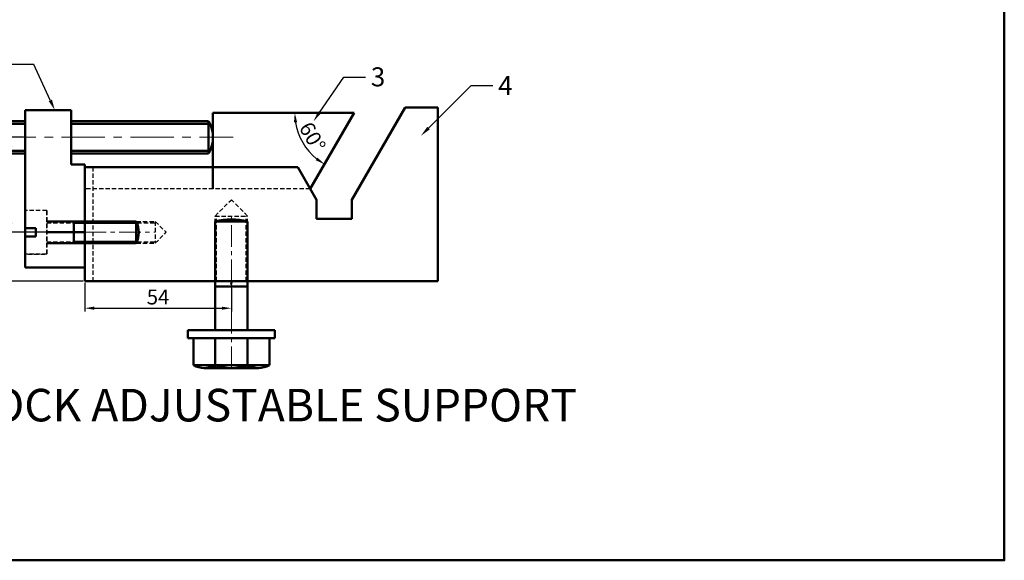
# Model space of a CAD drawing. Units: millimetres. Extents: x 10 to 613, y -226 to 271.
# Tile 2 of 4: x 251 to 613, y -226 to -26. Entities that reach past the tile are written whole.
import ezdxf
from ezdxf import colors
from ezdxf.entities.mleader import LeaderData, LeaderLine
from ezdxf.math import Vec2, Vec3

# ---------------------------------------------------------------- set-up
doc = ezdxf.new("R2010")
doc.units = ezdxf.units.MM
doc.header["$LTSCALE"] = 0.5
doc.linetypes.add('CENTER', pattern=[50.8, 31.75, -6.35, 6.35, -6.35])
doc.linetypes.add('HIDDEN', pattern=[9.525, 6.35, -3.175])
for name, color, linetype, lineweight in [('M-CNTR', 1, 'CENTER', 18), ('M-DIMS', 2, 'Continuous', 25), ('M-HIDN', 6, 'HIDDEN', 25), ('M-OUTL', 7, 'Continuous', 50), ('M-TEXT', 3, 'Continuous', 25), ('M-TTLB', 7, 'Continuous', 50)]:
    doc.layers.add(name, color=color, linetype=linetype, lineweight=lineweight)
doc.styles.get("Standard").update_dxf_attribs({"font": 'arial.ttf'})
doc.dimstyles.new('ISO-25', dxfattribs={"dimtxt": 5.5, "dimasz": 3.5, "dimexe": 1.25, "dimexo": 0.625, "dimtad": 1, "dimtoh": 1, "dimtxsty": 'Standard', "dimcen": 2.5, "dimadec": 0, "dimazin": 0, "dimtfac": 1, "dimtmove": 0, "dimatfit": 3, "dimfxl": 1, "dimarcsym": 0})

# ---------------------------------------------------------------- blocks, each defined once
blk = doc.blocks.new('*D52')
at = {"layer": 'Defpoints', "color": 0, "ltscale": 0.5, "transparency": 16777216}
for p in [(274.69, -104.71), (238.97, -122.71), (274.69, -122.71)]:
    blk.add_point(p, dxfattribs=at)
at = {"layer": 'M-DIMS', "color": 0, "lineweight": -2, "ltscale": 0.5, "transparency": 16777216}
for p, q in [((274.07, -104.71), (237.72, -104.71)), ((238.97, -108.21), (238.97, -119.21)), ((274.07, -122.71), (237.72, -122.71))]:
    blk.add_line(p, q, dxfattribs=at)
at = {"layer": 'M-DIMS', "color": 0, "ltscale": 0.5, "transparency": 16777216}
for points in [[(238.39, -108.21), (239.56, -108.21), (238.97, -104.71)], [(238.39, -119.21), (239.56, -119.21), (238.97, -122.71)]]:
    blk.add_solid(points, dxfattribs=at)
at = {"layer": 'M-DIMS', "color": 0, "ltscale": 0.5, "transparency": 16777216, "insert": (235.54, -113.71), "char_height": 5.5, "attachment_point": 5, "rotation": 90}
blk.add_mtext('18', dxfattribs=at)
blk = doc.blocks.new('*D53')
at = {"layer": 'Defpoints', "color": 0, "ltscale": 0.5, "transparency": 16777216}
for p in [(252.69, -69.71), (247.41, -104.71), (252.69, -104.71)]:
    blk.add_point(p, dxfattribs=at)
at = {"layer": 'M-DIMS', "color": 0, "lineweight": -2, "ltscale": 0.5, "transparency": 16777216}
for p, q in [((252.07, -69.71), (246.16, -69.71)), ((247.41, -73.21), (247.41, -101.21)), ((252.07, -104.71), (246.16, -104.71))]:
    blk.add_line(p, q, dxfattribs=at)
at = {"layer": 'M-DIMS', "color": 0, "ltscale": 0.5, "transparency": 16777216}
for points in [[(246.83, -73.21), (247.99, -73.21), (247.41, -69.71)], [(246.83, -101.21), (247.99, -101.21), (247.41, -104.71)]]:
    blk.add_solid(points, dxfattribs=at)
at = {"layer": 'M-DIMS', "color": 0, "ltscale": 0.5, "transparency": 16777216, "insert": (243.98, -87.21), "char_height": 5.5, "attachment_point": 5, "rotation": 90}
blk.add_mtext('35', dxfattribs=at)
blk = doc.blocks.new('*D54')
at = {"layer": 'Defpoints', "color": 0, "ltscale": 0.5, "transparency": 16777216}
for p in [(274.69, -122.71), (328.69, -124.69), (328.69, -132.66)]:
    blk.add_point(p, dxfattribs=at)
at = {"layer": 'M-DIMS', "color": 0, "lineweight": -2, "ltscale": 0.5, "transparency": 16777216}
for p, q in [((274.69, -123.33), (274.69, -133.91)), ((328.69, -125.31), (328.69, -133.91)), ((278.19, -132.66), (325.19, -132.66))]:
    blk.add_line(p, q, dxfattribs=at)
at = {"layer": 'M-DIMS', "color": 0, "ltscale": 0.5, "transparency": 16777216}
for points in [[(278.19, -132.08), (278.19, -133.24), (274.69, -132.66)], [(325.19, -132.08), (325.19, -133.24), (328.69, -132.66)]]:
    blk.add_solid(points, dxfattribs=at)
at = {"layer": 'M-DIMS', "color": 0, "ltscale": 0.5, "transparency": 16777216, "insert": (301.69, -129.24), "char_height": 5.5, "attachment_point": 5}
blk.add_mtext('54', dxfattribs=at)
blk = doc.blocks.new('*D55')
at = {"layer": 'Defpoints', "color": 0, "ltscale": 0.5, "transparency": 16777216}
for p in [(321.92, -60.71), (373.92, -60.71), (373.92, -60.71), (353.37, -68.19), (357.75, -88.71)]:
    blk.add_point(p, dxfattribs=at)
at = {"layer": 'M-DIMS', "color": 0, "lineweight": -2, "ltscale": 0.5, "transparency": 16777216}
blk.add_arc((373.92, -60.71), 21.87, 189.1792, 230.8208, dxfattribs=at)
at = {"layer": 'M-DIMS', "color": 0, "ltscale": 0.5, "transparency": 16777216}
for points in [[(351.75, -64.24), (352.91, -64.15), (352.05, -60.71)], [(360.43, -77.18), (359.77, -78.14), (362.98, -79.65)]]:
    blk.add_solid(points, dxfattribs=at)
at = {"layer": 'M-DIMS', "color": 0, "ltscale": 0.5, "transparency": 16777216, "insert": (357.95, -69.93), "char_height": 5.5, "attachment_point": 5, "rotation": 300}
blk.add_mtext('60°', dxfattribs=at)

msp = doc.modelspace()

# ---------------------------------------------------------------- linework, layer by layer
at = {"layer": 'M-CNTR'}
msp.add_line((215.384, -69.708), (329.34, -69.708), dxfattribs=at)
at = {"layer": 'M-CNTR', "ltscale": 0.5}
for p, q in [((328.691, -122.708), (328.691, -98.708)), ((274.691, -104.708), (300.691, -104.708)), ((328.691, -154.69), (328.691, -122.977))]:
    msp.add_line(p, q, dxfattribs=at)
at = {"layer": 'M-HIDN', "ltscale": 0.5}
for p, q in [((277.691, -80.708), (277.691, -122.708)), ((357.752, -88.708), (274.691, -88.708)), ((322.691, -98.708), (328.691, -92.708)), ((334.691, -98.708), (328.691, -92.708)), ((260.691, -96.708), (252.691, -96.708)), ((260.691, -96.708), (253.691, -96.708)), ((260.691, -96.708), (260.691, -112.708)), ((260.691, -112.708), (260.691, -96.708)), ((274.691, -100.708), (260.691, -100.708)), ((260.691, -101.208), (300.691, -101.208)), ((274.691, -100.708), (300.691, -100.708)), ((300.691, -100.708), (300.691, -108.708)), ((300.691, -100.708), (304.691, -104.708)), ((322.691, -122.708), (322.691, -98.708)), ((322.691, -98.708), (334.691, -98.708)), ((323.191, -122.708), (323.191, -98.708)), ((334.191, -122.708), (334.191, -98.708)), ((334.691, -122.708), (334.691, -98.708)), ((300.691, -108.708), (304.691, -104.708)), ((260.691, -108.208), (300.691, -108.208)), ((274.691, -108.708), (260.691, -108.708)), ((274.691, -108.708), (300.691, -108.708)), ((260.691, -112.708), (252.691, -112.708)), ((253.691, -112.708), (260.691, -112.708))]:
    msp.add_line(p, q, dxfattribs=at)
at = {"layer": 'M-OUTL', "ltscale": 0.5}
for p, q in [((269.691, -59.708), (252.691, -59.708)), ((252.691, -59.708), (252.691, -117.708)), ((269.691, -79.708), (269.691, -59.708)), ((321.918, -60.708), (321.918, -88.708)), ((321.918, -60.708), (373.918, -60.708)), ((373.918, -60.708), (357.752, -88.708)), ((404.691, -58.708), (392.691, -58.708)), ((404.691, -122.708), (404.691, -58.708)), ((274.691, -79.708), (269.691, -79.708)), ((274.691, -117.708), (274.691, -79.708)), ((274.691, -122.708), (274.691, -80.708)), ((274.691, -80.708), (353.133, -80.708)), ((252.691, -96.708), (252.691, -103.208)), ((293.691, -100.708), (260.691, -100.708)), ((270.691, -108.708), (270.691, -100.708)), ((293.691, -101.208), (270.691, -101.208)), ((293.691, -108.708), (293.691, -100.708)), ((328.691, -100.69), (322.691, -100.69)), ((322.691, -100.69), (322.691, -140.69)), ((328.691, -100.69), (334.691, -100.69)), ((334.691, -100.69), (334.691, -140.69)), ((252.691, -103.208), (256.691, -103.208)), ((256.691, -103.208), (256.691, -106.208)), ((260.691, -104.708), (274.691, -104.708)), ((252.691, -106.208), (252.691, -112.708)), ((256.691, -106.208), (252.691, -106.208)), ((293.691, -108.708), (260.691, -108.708)), ((293.691, -108.208), (270.691, -108.208)), ((252.691, -117.708), (274.691, -117.708)), ((404.691, -122.708), (274.691, -122.708)), ((328.691, -122.977), (328.678, -123.977)), ((379.497, -122.708), (404.691, -122.708)), ((322.691, -124.69), (334.691, -124.69)), ((312.691, -140.69), (344.691, -140.69)), ((312.691, -143.69), (312.691, -140.69)), ((344.691, -140.69), (344.691, -143.69)), ((344.691, -143.69), (312.691, -143.69)), ((314.691, -143.69), (342.691, -143.69)), ((314.691, -153.69), (314.691, -143.69)), ((322.691, -143.69), (322.691, -154.69)), ((334.691, -143.69), (334.691, -154.69)), ((342.691, -143.69), (342.691, -153.69)), ((342.691, -153.69), (314.691, -153.69)), ((338.815, -154.69), (318.567, -154.69))]:
    msp.add_line(p, q, dxfattribs=at)
at = {"layer": 'M-OUTL'}
for p, q in [((252.691, -63.708), (240.31, -63.708)), ((252.691, -64.708), (240.31, -64.708)), ((320.31, -63.708), (269.691, -63.708)), ((320.31, -64.708), (269.691, -64.708)), ((320.31, -69.708), (320.31, -63.708)), ((320.31, -69.708), (320.31, -75.708)), ((252.691, -74.708), (240.31, -74.708)), ((252.691, -75.708), (240.31, -75.708)), ((320.31, -74.708), (269.691, -74.708)), ((320.31, -75.708), (269.691, -75.708))]:
    msp.add_line(p, q, dxfattribs=at)
at = {"layer": 'M-OUTL', "ltscale": 0.5}
msp.add_lwpolyline([(353.133, -80.708), (360.062, -92.708), (360.062, -99.708), (373.062, -99.708), (373.062, -92.708), (392.691, -58.708)], dxfattribs=at)
for centre, radius, start, end in [((309.918, -69.708), 12, 330, 30), ((285.332, -104.708), 9.267, 334.42974, 25.57026), ((328.691, -124.256), 24.318, 75.71605, 104.28395), ((318.691, -146.197), 8.493, 241.90309, 298.09691), ((328.691, -136.19), 18.5, 251.07536, 288.92464), ((338.691, -146.197), 8.493, 241.90309, 298.09691)]:
    msp.add_arc(centre, radius, start, end, dxfattribs=at)
at = {"layer": 'M-TTLB', "ltscale": 0.5}
msp.add_lwpolyline([(9.692, 270.659), (613.416, 270.659), (613.416, -225.522), (9.692, -225.522)], close=True, dxfattribs=at)

# ---------------------------------------------------------------- texts
at = {"layer": 'M-TEXT', "ltscale": 0.5, "insert": (207.538, -162.361), "char_height": 12, "attachment_point": 1}
msp.add_mtext_dynamic_manual_height_columns('V BLOCK ADJUSTABLE SUPPORT', width=297.62232, gutter_width=12.5, heights=[0], dxfattribs=at)

# ---------------------------------------------------------------- dimensions: what is measured, and where the dimension line sits
at = {"layer": 'M-DIMS', "ltscale": 0.5}
dim = msp.add_angular_dim_2l(base=(353.367, -68.188), line1=((373.918, -60.708), (357.752, -88.708)), line2=((321.918, -60.708), (373.918, -60.708)), dimstyle='ISO-25', override={"dimclrd": 0, "dimclre": 0, "dimclrt": 0}, dxfattribs=at)
dim.commit()
dim.dimension.update_dxf_attribs({"geometry": '*D55', "text_midpoint": (357.951, -69.926)})
for base, p1, p2, picture, middle in [((247.411, -104.708), (252.691, -69.708), (252.691, -104.708), '*D53', (243.976, -87.208)), ((238.972, -122.708), (274.691, -104.708), (274.691, -122.708), '*D52', (235.539, -113.708))]:
    dim = msp.add_linear_dim(base=base, p1=p1, p2=p2, angle=90, dimstyle='ISO-25', override={"dimclrd": 0, "dimclre": 0, "dimclrt": 0}, dxfattribs=at)
    dim.commit()
    dim.dimension.update_dxf_attribs({"geometry": picture, "text_midpoint": middle})
dim = msp.add_linear_dim(base=(328.691, -132.661), p1=(274.691, -122.708), p2=(328.691, -124.69), dimstyle='ISO-25', override={"dimclrd": 0, "dimclre": 0, "dimclrt": 0}, dxfattribs=at)
dim.commit()
dim.dimension.update_dxf_attribs({"geometry": '*D54', "text_midpoint": (301.691, -129.239)})

# ---------------------------------------------------------------- leaders
ml = msp.add_multileader_mtext('Standard', dxfattribs=at)
ml.set_content('2', color=256)
ml.set_leader_properties()
ml.build(insert=Vec2(0, 0))
ctx = ml.context
ctx.base_point, ctx.char_height, ctx.plane_origin = Vec3(239.253, -42.893), 7, Vec3(263.676, -59.708)
ctx.text_align_type = 2
notes = []
notes.append((ctx, [(0, (1, 1, 0), (255.89, -42.893), (-1, 0), 8, [(0, [(263.676, -59.708)], 0, [])])]))
ctx.mtext.insert, ctx.mtext.alignment, ctx.mtext.flow_direction = Vec3(245.89, -39.393), 3, 5
ml = msp.add_multileader_mtext('Standard', dxfattribs=at)
ml.set_content('3', color=256)
ml.set_leader_properties()
ml.build(insert=Vec2(0, 0))
ctx = ml.context
ctx.base_point, ctx.char_height, ctx.plane_origin = Vec3(378.08, -47.506), 7, Vec3(358.943, -63.826)
notes.append((ctx, [(0, (1, 1, 0), (370.08, -47.506), (1, 0), 8, [(0, [(358.943, -63.826)], 0, [])])]))
ctx.mtext.insert, ctx.mtext.flow_direction = Vec3(380.08, -43.944), 5
ml = msp.add_multileader_mtext('Standard', dxfattribs=at)
ml.set_content('4', color=256)
ml.set_leader_properties()
ml.build(insert=Vec2(0, 0))
ctx = ml.context
ctx.base_point, ctx.char_height, ctx.plane_origin = Vec3(424.979, -50.675), 7, Vec3(398.501, -69.153)
notes.append((ctx, [(0, (1, 1, 0), (416.979, -50.675), (1, 0), 8, [(0, [(398.501, -69.153)], 0, [])])]))
ctx.mtext.insert, ctx.mtext.flow_direction = Vec3(426.979, -47.175), 5
for ctx, leaders in notes:
    for number, flags, end, landing, length, lines in leaders:
        leader = LeaderData()
        leader.index, (leader.has_last_leader_line, leader.has_dogleg_vector, leader.attachment_direction) = number, flags
        leader.last_leader_point, leader.dogleg_vector, leader.dogleg_length = Vec3(end), Vec3(landing), length
        for number, points, colour, breaks in lines:
            line = LeaderLine()
            line.index, line.vertices, line.color, line.breaks = number, Vec3.list(points), colors.encode_raw_color(colour), breaks
            leader.lines.append(line)
        ctx.leaders.append(leader)

doc.saveas('drawing.dxf')
